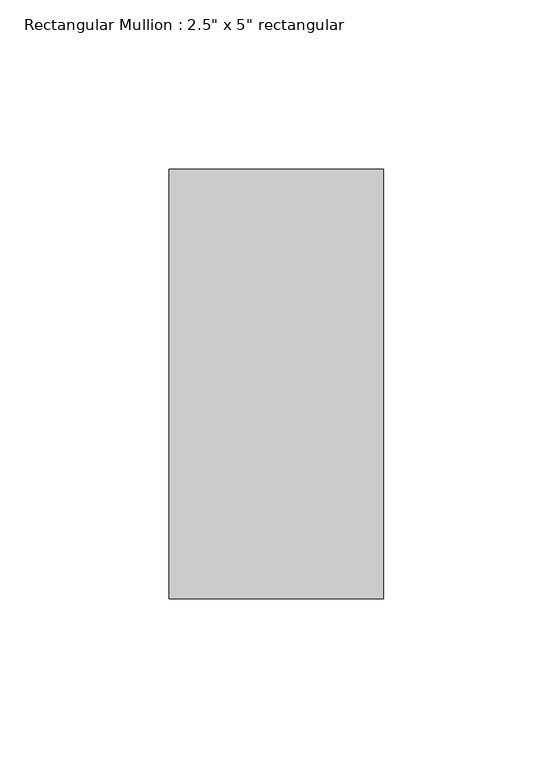
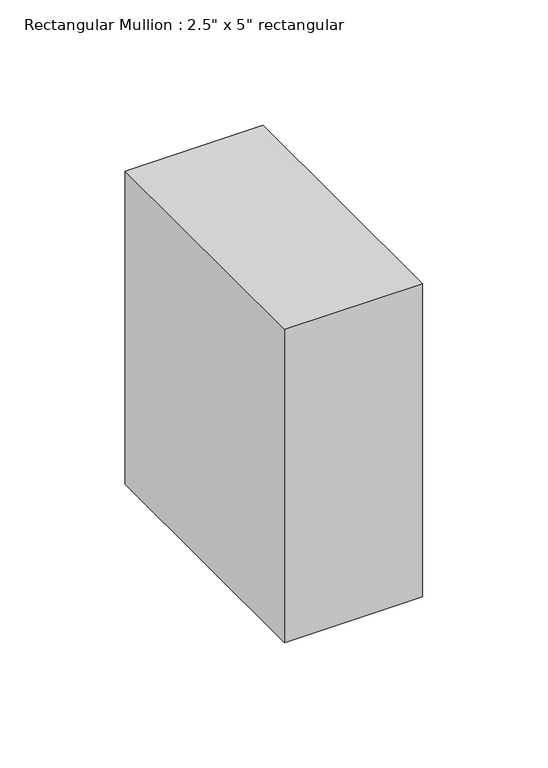
"""IFC4 building model written with IfcOpenShell, lengths in millimetres: member geometry."""

from ifc_helpers import new_model, si_unit, frame, origin, place, context, project, spatial, polyline, outline, extrude, source, transform, mapped, element, save


def member_f6f0dfdd(model_context):
    return source(origin(), model_context, "Body", "SweptSolid", [
        extrude(outline(polyline([(31.75, 63.5), (31.75, -63.5), (-31.75, -63.5), (-31.75, 63.5), (31.75, 63.5)])), frame((0.0, 0.0, -152.4), z_axis=(0.0, 0.0, 1.0), x_axis=(1.0, 0.0, 0.0)), (0.0, 0.0, 1.0), 152.4),
    ])


if __name__ == "__main__":
    model = new_model("IFC4")
    model_context = context("Model", 3, world=origin())
    ifc_project = project(units=[si_unit("LENGTHUNIT", "METRE", prefix="MILLI")], contexts=[model_context])
    site = spatial("IfcSite", under=ifc_project)
    building = spatial("IfcBuilding", under=site)
    placement = place(None, origin())
    member_shape = member_f6f0dfdd(model_context)
    element("IfcMember", 1, ObjectType="Rectangular Mullion : 2.5\" x 5\" rectangular", at=placement, inside=building, context=model_context, shape_type="MappedRepresentation", body=[
        mapped(member_shape, transform((0.0, 0.0, 0.0), x_axis=(1.0, 0.0, 0.0), y_axis=(0.0, 1.0, 0.0), z_axis=(0.0, 0.0, 1.0))),
    ])
    save(model, "model.ifc")

# Revit data of these elements
# Type "Rectangular Mullion : 2.5\" x 5\" rectangular"
#   built-in parameter 1007304 = 0.416667 (stored number, unit not read)
#   built-in parameter 1007301 = 0.104167 (stored number, unit not read)
#   built-in parameter 1007300 = 0.104167 (stored number, unit not read)
# Element 1 (IfcMember, "Rectangular Mullion : 2.5\" x 5\" rectangular")
#   Materials on its faces: "Aluminum"
# Materials
#   "Aluminum": class "Metal", colour RGB 247 247 247, transparency 0, Description = "Aluminum 6061", Cost = 0
